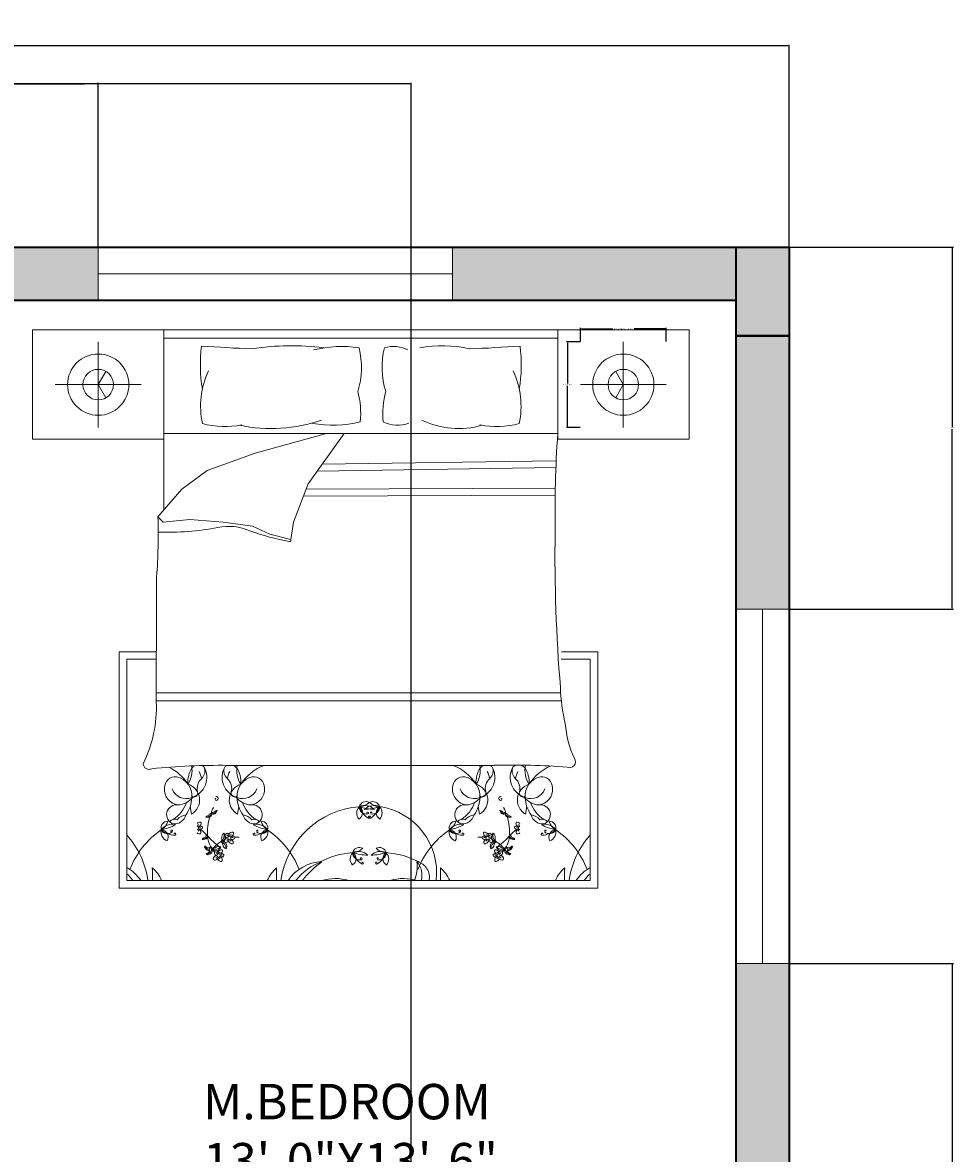
# Model space of a CAD drawing. Units: inches. Extents: x -10 to 455, y -513 to 57.
# Tile 4 of 4: x 297 to 455, y -134 to 57. Entities that reach past the tile are written whole.
import ezdxf

# ---------------------------------------------------------------- set-up
doc = ezdxf.new("R2010")
doc.units = ezdxf.units.IN
doc.header["$MEASUREMENT"] = 0
for name, color, linetype, lineweight in [('A-ANNO-DIMS', 2, 'Continuous', 18), ('A-AREA-IDEN', 7, 'Continuous', 18), ('A-COLS', 7, 'Continuous', 40), ('A-COLS-PATT', 1, 'Continuous', 13), ('A-FURN', 8, 'Continuous', 13), ('A-GLAZ', 222, 'Continuous', 18), ('A-WALL', 7, 'Continuous', 35), ('A-WALL-PATT', 152, 'Continuous', 13)]:
    doc.layers.add(name, color=color, linetype=linetype, lineweight=lineweight)
doc.styles.get("Standard").update_dxf_attribs({"font": 'arial.ttf'})
doc.dimstyles.get("Standard").update_dxf_attribs({"dimtxt": 0.18, "dimasz": 0.18, "dimexe": 0.18, "dimexo": 0.0625, "dimgap": 0.09, "dimtad": 0, "dimtih": 1, "dimtoh": 1, "dimdec": 0, "dimzin": 0, "dimdsep": 46, "dimlunit": 3, "dimtxsty": 'Standard', "dimcen": 0.09, "dimadec": 0, "dimazin": 0, "dimtfac": 1, "dimtdec": 0, "dimtofl": 0, "dimtmove": 0, "dimatfit": 3, "dimfxl": 1, "dimtolj": 1, "dimtzin": 0, "dimarcsym": 0})

# ---------------------------------------------------------------- blocks, each defined once
blk = doc.blocks.new('*D1')
at = {"layer": 'A-ANNO-DIMS', "color": 0, "lineweight": -2, "transparency": 16777216}
for p, q in [((40.25, 19.21), (40.25, 53.43)), ((40.43, 53.25), (223.35, 53.25)), ((427.07, 53.25), (244.14, 53.25)), ((427.25, 19.21), (427.25, 53.43))]:
    blk.add_line(p, q, dxfattribs=at)
at = {"layer": 'A-ANNO-DIMS', "color": 0, "transparency": 16777216}
for points in [[(40.43, 53.28), (40.43, 53.22), (40.25, 53.25)], [(427.07, 53.28), (427.07, 53.22), (427.25, 53.25)]]:
    blk.add_solid(points, dxfattribs=at)
at = {"layer": 'Defpoints', "color": 0, "transparency": 16777216}
for p in [(427.25, 53.25), (40.25, 19.15), (427.25, 19.15)]:
    blk.add_point(p, dxfattribs=at)
at = {"layer": 'A-ANNO-DIMS', "color": 0, "transparency": 16777216, "insert": (233.75, 53.25), "char_height": 6, "attachment_point": 5}
blk.add_mtext('\\A1;32\'-3"', dxfattribs=at)
blk = doc.blocks.new('WIN-60IN')
for p, q in [((0, 9), (60, 9)), ((0, 0), (0, 9)), ((60, 9), (60, 0)), ((0, 4.5), (60, 4.5)), ((60, 0), (0, 0))]:
    blk.add_line(p, q)
blk = doc.blocks.new('LAMP-BEDSIDE-LARGE')
for p, q in [((7.26, 0), (7.26, 14.53)), ((0, 7.26), (14.53, 7.26))]:
    blk.add_line(p, q)
for points in [[(7.26, 7.26), (5.97, 9.51)], [(7.26, 7.26), (5.97, 5.02)]]:
    blk.add_lwpolyline(points)
for radius in [5.19, 2.59]:
    blk.add_circle((7.26, 7.26), radius)
blk = doc.blocks.new('*D26')
at = {"layer": 'A-ANNO-DIMS', "color": 0, "lineweight": -2, "transparency": 16777216}
for p, q in [((391.92, 3.2), (391.92, 5.5)), ((392.1, 5.32), (397.38, 5.32)), ((406.27, 5.32), (401, 5.32)), ((406.45, 3.2), (406.45, 5.5))]:
    blk.add_line(p, q, dxfattribs=at)
at = {"layer": 'A-ANNO-DIMS', "color": 0, "transparency": 16777216}
for points in [[(392.1, 5.35), (392.1, 5.29), (391.92, 5.32)], [(406.27, 5.35), (406.27, 5.29), (406.45, 5.32)]]:
    blk.add_solid(points, dxfattribs=at)
at = {"layer": 'Defpoints', "color": 0, "transparency": 16777216}
for p in [(406.45, 5.32), (391.92, 3.14), (406.45, 3.14)]:
    blk.add_point(p, dxfattribs=at)
at = {"layer": 'A-ANNO-DIMS', "color": 0, "transparency": 16777216, "insert": (399.19, 5.32), "char_height": 0.18, "attachment_point": 5}
blk.add_mtext('\\A1;BEDSIDE LAMP 1\'-2 1/2" TYP.', dxfattribs=at)
blk = doc.blocks.new('*D27')
at = {"layer": 'A-ANNO-DIMS', "color": 0, "lineweight": -2, "transparency": 16777216}
for p, q in [((391.86, 3.14), (389.56, 3.14)), ((389.74, 2.96), (389.74, -3.94)), ((389.74, -11.21), (389.74, -4.31)), ((391.86, -11.39), (389.56, -11.39))]:
    blk.add_line(p, q, dxfattribs=at)
at = {"layer": 'A-ANNO-DIMS', "color": 0, "transparency": 16777216}
for points in [[(389.71, 2.96), (389.77, 2.96), (389.74, 3.14)], [(389.71, -11.21), (389.77, -11.21), (389.74, -11.39)]]:
    blk.add_solid(points, dxfattribs=at)
at = {"layer": 'Defpoints', "color": 0, "transparency": 16777216}
for p in [(389.74, 3.14), (391.92, 3.14), (391.92, -11.39)]:
    blk.add_point(p, dxfattribs=at)
at = {"layer": 'A-ANNO-DIMS', "color": 0, "transparency": 16777216, "insert": (389.74, -4.12), "char_height": 0.18, "attachment_point": 5}
blk.add_mtext('\\A1;1\'-2 1/2" TYP.', dxfattribs=at)
blk = doc.blocks.new('*D32')
at = {"layer": 'A-ANNO-DIMS', "color": 0, "lineweight": -2, "transparency": 16777216}
for p, q in [((237.5, 19.21), (237.5, 46.98)), ((237.68, 46.8), (273.54, 46.8)), ((310.07, 46.8), (274.2, 46.8)), ((310.25, 19.21), (310.25, 46.98))]:
    blk.add_line(p, q, dxfattribs=at)
at = {"layer": 'A-ANNO-DIMS', "color": 0, "transparency": 16777216}
for points in [[(237.68, 46.83), (237.68, 46.77), (237.5, 46.8)], [(310.07, 46.83), (310.07, 46.77), (310.25, 46.8)]]:
    blk.add_solid(points, dxfattribs=at)
at = {"layer": 'Defpoints', "color": 0, "transparency": 16777216}
for p in [(310.25, 46.8), (237.5, 19.15), (310.25, 19.15)]:
    blk.add_point(p, dxfattribs=at)
at = {"layer": 'A-ANNO-DIMS', "color": 0, "transparency": 16777216, "insert": (273.87, 46.8), "char_height": 0.18, "attachment_point": 5}
blk.add_mtext('\\A1;6\'-1"', dxfattribs=at)
blk = doc.blocks.new('*D37')
at = {"layer": 'A-ANNO-DIMS', "color": 0, "lineweight": -2, "transparency": 16777216}
for p, q in [((427.31, 19.15), (455.08, 19.15)), ((454.9, 18.97), (454.9, -11.33)), ((454.9, -41.99), (454.9, -11.69)), ((427.31, -42.17), (455.08, -42.17))]:
    blk.add_line(p, q, dxfattribs=at)
at = {"layer": 'A-ANNO-DIMS', "color": 0, "transparency": 16777216}
for points in [[(454.87, 18.97), (454.93, 18.97), (454.9, 19.15)], [(454.87, -41.99), (454.93, -41.99), (454.9, -42.17)]]:
    blk.add_solid(points, dxfattribs=at)
at = {"layer": 'Defpoints', "color": 0, "transparency": 16777216}
for p in [(427.25, 19.15), (427.25, -42.17), (454.9, -42.17)]:
    blk.add_point(p, dxfattribs=at)
at = {"layer": 'A-ANNO-DIMS', "color": 0, "transparency": 16777216, "insert": (454.9, -11.51), "char_height": 0.18, "attachment_point": 5}
blk.add_mtext('\\A1;5\'-1 1/2"', dxfattribs=at)
blk = doc.blocks.new('*D38')
at = {"layer": 'A-ANNO-DIMS', "color": 0, "lineweight": -2, "transparency": 16777216}
for p, q in [((427.31, -102.17), (455.08, -102.17)), ((454.9, -102.35), (454.9, -188.62)), ((454.9, -275.26), (454.9, -188.98)), ((427.31, -275.44), (455.08, -275.44))]:
    blk.add_line(p, q, dxfattribs=at)
at = {"layer": 'A-ANNO-DIMS', "color": 0, "transparency": 16777216}
for points in [[(454.87, -102.35), (454.93, -102.35), (454.9, -102.17)], [(454.87, -275.26), (454.93, -275.26), (454.9, -275.44)]]:
    blk.add_solid(points, dxfattribs=at)
at = {"layer": 'Defpoints', "color": 0, "transparency": 16777216}
for p in [(427.25, -102.17), (427.25, -275.44), (454.9, -275.44)]:
    blk.add_point(p, dxfattribs=at)
at = {"layer": 'A-ANNO-DIMS', "color": 0, "transparency": 16777216, "insert": (454.9, -188.8), "char_height": 0.18, "attachment_point": 5}
blk.add_mtext('\\A1;14\'-5 1/2"', dxfattribs=at)
blk = doc.blocks.new('*D41')
at = {"layer": 'A-ANNO-DIMS', "color": 0, "lineweight": -2, "transparency": 16777216}
for p, q in [((253.25, -160.79), (253.25, 46.98)), ((253.43, 46.8), (307.92, 46.8)), ((363.07, 46.8), (308.58, 46.8)), ((363.25, -160.79), (363.25, 46.98))]:
    blk.add_line(p, q, dxfattribs=at)
at = {"layer": 'A-ANNO-DIMS', "color": 0, "transparency": 16777216}
for points in [[(253.43, 46.83), (253.43, 46.77), (253.25, 46.8)], [(363.07, 46.83), (363.07, 46.77), (363.25, 46.8)]]:
    blk.add_solid(points, dxfattribs=at)
at = {"layer": 'Defpoints', "color": 0, "transparency": 16777216}
for p in [(363.25, 46.8), (253.25, -160.85), (363.25, -160.85)]:
    blk.add_point(p, dxfattribs=at)
at = {"layer": 'A-ANNO-DIMS', "color": 0, "transparency": 16777216, "insert": (308.25, 46.8), "char_height": 0.18, "attachment_point": 5}
blk.add_mtext('\\A1;9\'-2"', dxfattribs=at)
blk = doc.blocks.new('*D45')
at = {"layer": 'A-ANNO-DIMS', "color": 0, "lineweight": -2, "transparency": 16777216}
for p, q in [((257.66, -111.85), (257.84, -111.85)), ((257.75, -111.94), (257.75, -111.76)), ((300.74, -154.84), (284.74, -138.85)), ((300.92, -154.84), (300.74, -154.84))]:
    blk.add_line(p, q, dxfattribs=at)
at = {"layer": 'A-ANNO-DIMS', "color": 0, "transparency": 16777216}
blk.add_solid([(284.76, -138.83), (284.72, -138.87), (284.62, -138.72)], dxfattribs=at)
at = {"layer": 'Defpoints', "color": 0, "transparency": 16777216}
for p in [(257.75, -111.85), (284.62, -138.72)]:
    blk.add_point(p, dxfattribs=at)
at = {"layer": 'A-ANNO-DIMS', "color": 0, "transparency": 16777216, "insert": (301.33, -154.84), "char_height": 0.18, "attachment_point": 5}
blk.add_mtext('\\A1;R3\'-2"', dxfattribs=at)

msp = doc.modelspace()

# ---------------------------------------------------------------- hatches: boundary and pattern name
at = {"layer": 'A-COLS-PATT'}
h = msp.add_hatch(color=256, dxfattribs=at)
h.dxf.hatch_style = 1
h.paths.add_polyline_path([(55.25, 19.15), (40.25, 19.15), (40.25, 10.15), (55.25, 10.15)])
h.paths.add_polyline_path([(262.25, 19.15), (253.25, 19.15), (253.25, 4.15), (262.25, 4.15)])
h.paths.add_polyline_path([(427.25, 19.15), (418.25, 19.15), (418.25, 4.15), (427.25, 4.15)])
h.paths.add_polyline_path([(427.25, -247.85), (418.25, -247.85), (418.25, -262.85), (427.25, -262.85)])
h.paths.add_polyline_path([(268.25, -247.85), (253.25, -247.85), (253.25, -256.85), (268.25, -256.85)])
h.paths.add_polyline_path([(55.25, -247.85), (40.25, -247.85), (40.25, -256.85), (55.25, -256.85)])
h.paths.add_polyline_path([(55.25, -475.85), (49.25, -475.85), (40.25, -475.85), (40.25, -484.85), (55.25, -484.85)])
h.paths.add_polyline_path([(268.25, -475.85), (253.25, -475.85), (253.25, -484.85), (268.25, -484.85)])
h.paths.add_polyline_path([(427.25, -469.85), (418.25, -469.85), (418.25, -484.85), (427.25, -484.85)])
h.paths.add_polyline_path([(55.25, -100.85), (40.25, -100.85), (40.25, -109.85), (55.25, -109.85)])
at = {"layer": 'A-WALL-PATT'}
h = msp.add_hatch(color=256, dxfattribs=at)
h.dxf.hatch_style = 1
h.paths.add_polyline_path([(418.25, -151.85), (268.25, -151.85), (268.25, -160.85), (418.25, -160.85)])
h.paths.add_polyline_path([(165.25, -100.85), (55.25, -100.85), (55.25, -109.85), (165.25, -109.85), (165.25, -105.35)])
h.paths.add_polyline_path([(49.25, -75.35), (40.25, -75.35), (40.25, -100.85), (49.25, -100.85)])
h.paths.add_polyline_path([(49.25, 10.15), (40.25, 10.15), (40.25, -15.35), (49.25, -15.35)])
h.paths.add_polyline_path([(86.75, 19.15), (55.25, 19.15), (55.25, 10.15), (86.75, 10.15)])
h.paths.add_polyline_path([(213.5, 19.15), (146.75, 19.15), (146.75, 10.15), (193.25, 10.15), (193.25, -28.04), (197.75, -28.04), (197.75, 10.15), (213.5, 10.15)])
h.paths.add_polyline_path([(262.25, 4.15), (253.25, 4.15), (253.25, -69.35), (197.75, -69.35), (197.75, -60), (193.25, -60), (193.25, -109.85), (197.75, -109.85), (197.75, -73.85), (253.25, -73.85), (253.25, -109.85), (262.25, -109.85)])
h.paths.add_polyline_path([(310.25, 19.15), (262.25, 19.15), (262.25, 10.15), (310.25, 10.15)])
h.paths.add_polyline_path([(253.25, 19.15), (237.5, 19.15), (237.5, 10.15), (253.25, 10.15)])
h.paths.add_polyline_path([(418.25, 19.15), (370.25, 19.15), (370.25, 10.15), (418.25, 10.15)])
h.paths.add_polyline_path([(427.25, 4.15), (418.25, 4.15), (418.25, -42.17), (427.25, -42.17)])
h.paths.add_polyline_path([(427.25, -102.17), (418.25, -102.17), (418.25, -145.85), (427.25, -145.85)])
h.paths.add_polyline_path([(427.25, -160.85), (418.25, -160.85), (418.25, -247.85), (427.25, -247.85)])
h.paths.add_polyline_path([(418.25, -247.85), (365.75, -247.85), (365.75, -256.85), (418.25, -256.85)], flags=17)
h.paths.add_polyline_path([(297.25, -247.85), (268.25, -247.85), (268.25, -256.85), (297.25, -256.85), (297.25, -252.35)], flags=17)
h.paths.add_polyline_path([(427.25, -299.44), (418.25, -299.44), (418.25, -319.85), (370.25, -319.85), (370.25, -284.85), (368, -284.85), (365.75, -284.85), (365.75, -319.85), (329.75, -319.85), (329.75, -247.85), (325.25, -247.85), (325.25, -319.85), (257.75, -319.85), (257.75, -256.85), (253.25, -256.85), (253.25, -324.35), (262.25, -324.35), (418.25, -324.35), (418.25, -363.39), (427.25, -363.39)])
h.paths.add_polyline_path([(262.25, -352.35), (257.75, -352.35), (253.25, -352.35), (253.25, -447.85), (257.75, -447.85), (262.25, -447.85)])
h.paths.add_polyline_path([(305.75, -475.85), (268.25, -475.85), (268.25, -484.85), (305.75, -484.85)])
h.paths.add_polyline_path([(418.25, -475.85), (365.75, -475.85), (365.75, -484.85), (418.25, -484.85)])
h.paths.add_polyline_path([(427.25, -423.39), (418.25, -423.39), (418.25, -469.85), (427.25, -469.85)])
h.paths.add_polyline_path([(202.25, -247.85), (193.25, -247.85), (193.25, -403.85), (49.25, -403.85), (49.25, -360.35), (40.25, -360.35), (40.25, -412.85), (202.25, -412.85)])
h.paths.add_polyline_path([(165.25, -247.85), (55.25, -247.85), (55.25, -256.85), (165.25, -256.85), (165.25, -252.35)], flags=17)
h.paths.add_polyline_path([(49.25, -225.11), (40.25, -225.11), (40.25, -247.85), (49.25, -247.85)])
h.paths.add_polyline_path([(49.25, -256.85), (40.25, -256.85), (40.25, -300.35), (49.25, -300.35)], flags=17)
h.paths.add_polyline_path([(49.25, -137.85), (44.75, -137.85), (40.25, -137.85), (40.25, -165.11), (49.25, -165.11)])

# ---------------------------------------------------------------- linework, layer by layer
at = {"layer": 'A-COLS'}
msp.add_line((418.25, 4.15), (427.25, 4.15), dxfattribs=at)
at = {"layer": 'A-FURN'}
for p, q in [((299.12, 5.14), (410.31, 5.14)), ((321.35, 5.14), (321.35, -25.38)), ((388.07, 3.72), (321.35, 3.72)), ((321.35, -12.43), (388.07, -12.43)), ((336.8, -15.73), (348.92, -12.43)), ((351.9, -12.43), (345.81, -20.91)), ((328.69, -18.66), (336.8, -15.73)), ((387.77, -17.05), (348.18, -17.6)), ((324.41, -21.81), (328.69, -18.66)), ((387.73, -18.19), (347.35, -18.76)), ((345.81, -20.91), (343.33, -27.44)), ((320.36, -26.54), (324.41, -21.81)), ((387.68, -22.83), (345.01, -23.01)), ((387.67, -21.69), (345.45, -21.86)), ((321.26, -27.44), (320.36, -26.54)), ((325.76, -26.99), (321.26, -27.44)), ((331.39, -27.44), (325.76, -26.99)), ((336.35, -28.11), (331.39, -27.44)), ((339.28, -29.46), (336.35, -28.11)), ((343.33, -27.44), (342.88, -30.36)), ((342.88, -30.36), (339.28, -29.46)), ((313.79, -49.36), (320.08, -49.36)), ((313.79, -89.42), (313.79, -49.36)), ((388.69, -49.36), (394.86, -49.36)), ((394.86, -49.36), (394.86, -89.42)), ((320.08, -50.65), (315.08, -50.65)), ((315.08, -50.65), (315.08, -88.13)), ((393.57, -50.65), (388.67, -50.65)), ((393.57, -88.13), (393.57, -50.65)), ((388.57, -56.3), (320.07, -56.3)), ((388.68, -57.69), (320.07, -57.69)), ((377.28, -68.61), (332.14, -68.61)), ((326.04, -76.86), (325.79, -75.6)), ((333.81, -76.86), (334.05, -75.6)), ((374.84, -76.86), (374.59, -75.6)), ((382.61, -76.86), (382.86, -75.6)), ((394.86, -89.42), (313.79, -89.42)), ((315.08, -88.13), (393.57, -88.13))]:
    msp.add_line(p, q, dxfattribs=at)
for points in [[(321.35, -13.39), (299.12, -13.39), (299.12, 5.14)], [(388.07, 5.14), (388.07, -13.39), (410.31, -13.39), (410.31, 5.14)]]:
    msp.add_lwpolyline(points, dxfattribs=at)
for points in [[(327.74, 2.37, 0.074897), (327.88, -4.89, -0.472817)], [(354.19, -5.3, 0.14099), (354.41, 2.11, 0.235245)], [(358.94, -5.3, -0.14099), (358.72, 2.11, -0.235245)], [(381.68, 2.37, -0.074897), (381.55, -4.89, 0.472817)], [(320.13, -36.72, 0.001242), (320.07, -57.82, -0.127202), (317.84, -68.33)], [(388.54, -55.42, 0.056112), (389.35, -61.54, 0.095341), (390.91, -67.43)]]:
    msp.add_lwpolyline(points, format="xyb", dxfattribs=at)
for centre in [(332.46, -80.89), (376.19, -80.89), (330.61, -83.87), (378.04, -83.87)]:
    msp.add_circle(centre, 0.283, dxfattribs=at)
for centre, radius, start, end in [((389.03, 1060.56), 1059.96, 266.68521, 267.14978), ((342.98, -37.86), 40.33, 82.2196, 99.497), ((351.49, -17.48), 19.81, 81.5249, 103.96), ((360.24, -3.17), 5.5, 63.3437, 106.1026), ((368.49, -17.08), 19.55, 76.3427, 101.1841), ((320.39, 1060.56), 1059.96, 272.85022, 273.31479), ((341.91, -7.81), 14.33, 155.1316, 191.7583), ((367.52, -7.81), 14.33, 348.2417, 24.8684), ((341.08, -9.01), 13.62, 354.0129, 15.8293), ((372.05, -9.01), 13.62, 164.1707, 185.9871), ((331.71, 3.67), 14.9, 255.1039, 281.0369), ((339.55, 14.27), 25.84, 258.0397, 289.2615), ((350.01, 8.62), 19.61, 259.8617, 283.6238), ((360.99, -5.09), 5.89, 245.0183, 288.5407), ((371.29, 2.58), 14.15, 243.8761, 286.1746), ((377.72, 3.67), 14.9, 258.9631, 284.8961), ((587.4, -26.02), 199.79, 176.1, 180.9282), ((218.41, -29.3), 101.99, 355.8294, 1.553), ((322.26, 12.84), 41.97, 267.4519, 281.3392), ((332.29, -37.18), 9.05, 66.2616, 101.3392), ((350.6, 11.66), 43.12, 250.1194, 259.3383), ((342.63, -30.45), 0.268, 268.8623, 19.7536), ((648.22, -33.28), 260.62, 179.1145, 184.8735), ((318.87, -68.26), 1.03, 183.98, 297.3412), ((330.81, -184.35), 115.75, 89.3433, 95.6887), ((318.43, -76.44), 8.42, 33.6671, 63.2997), ((321.52, -69.43), 4.61, 328.8218, 9.1554), ((327.23, -69.84), 1.34, 120.0293, 142.325), ((325.09, -70.63), 3.54, 289.2822, 29.1751), ((326.66, -69.57), 1.66, 311.5653, 23.8354), ((327.23, -69.84), 1.34, 44.4517, 63.558), ((334.76, -70.63), 3.54, 150.8249, 250.7178), ((333.19, -69.57), 1.66, 156.1646, 228.4347), ((332.62, -69.84), 1.34, 113.229, 135.5483), ((332.62, -69.84), 1.34, 37.675, 66.7144), ((338.33, -69.43), 4.61, 169.7133, 211.1782), ((341.41, -76.44), 8.42, 111.4941, 146.3329), ((367.23, -76.44), 8.42, 33.6671, 68.5059), ((370.32, -69.43), 4.61, 328.8218, 10.2867), ((376.03, -69.84), 1.34, 113.2856, 142.325), ((373.89, -70.63), 3.54, 289.2822, 29.1751), ((376.03, -69.84), 1.34, 44.4517, 66.7144), ((375.46, -69.57), 1.66, 311.5653, 23.8354), ((380.69, -176.75), 108.2, 85.2402, 91.8035), ((383.56, -70.63), 3.54, 150.8249, 250.7178), ((381.99, -69.57), 1.66, 156.1646, 228.4347), ((381.42, -69.84), 1.34, 106.6343, 135.5483), ((381.42, -69.84), 1.34, 37.675, 72.5814), ((387.13, -69.43), 4.61, 169.249, 211.1782), ((390.21, -76.44), 8.42, 113.6453, 146.3329), ((390.07, -68), 1.01, 246.5219, 33.8264), ((323.34, -72.4), 1.88, 84.4856, 181.0538), ((322.76, -73.79), 3.34, 355.2933, 76.921), ((329.71, -71.43), 4.29, 145.785, 184.7304), ((329.28, -72.52), 2.28, 131.5653, 195.1471), ((324.55, -71.27), 3.2, 7.436, 29.9149), ((330.57, -72.52), 2.28, 344.8529, 48.4347), ((335.29, -71.27), 3.2, 150.0851, 172.564), ((330.13, -71.43), 4.29, 355.2696, 34.215), ((337.09, -73.79), 3.34, 103.079, 184.7067), ((336.51, -72.4), 1.88, 358.9462, 95.5144), ((372.14, -72.4), 1.88, 84.4856, 181.0538), ((371.56, -73.79), 3.34, 355.2933, 76.921), ((378.51, -71.43), 4.29, 145.785, 184.7304), ((378.08, -72.52), 2.28, 131.5653, 195.1471), ((373.35, -71.27), 3.2, 7.436, 29.9149), ((379.37, -72.52), 2.28, 344.8529, 48.4347), ((384.09, -71.27), 3.2, 150.0851, 172.564), ((378.94, -71.43), 4.29, 355.2696, 34.215), ((385.89, -73.79), 3.34, 103.079, 184.7067), ((385.31, -72.4), 1.88, 358.9462, 95.5144), ((324.11, -72.67), 2.66, 174.9449, 262.8857), ((325.15, -71.66), 2.58, 201.5819, 291.4221), ((324.66, -74.46), 2.76, 299.9085, 73.1337), ((335.19, -74.46), 2.76, 106.8663, 240.0915), ((334.7, -71.66), 2.58, 248.5779, 338.4181), ((335.74, -72.67), 2.66, 277.1143, 5.0551), ((372.91, -72.67), 2.66, 174.9449, 262.8857), ((373.95, -71.66), 2.58, 201.5819, 291.4221), ((373.46, -74.46), 2.76, 299.9085, 73.1337), ((383.99, -74.46), 2.76, 106.8663, 240.0915), ((383.5, -71.66), 2.58, 248.5779, 338.4181), ((384.54, -72.67), 2.66, 277.1143, 5.0551), ((323.64, -72.08), 3.23, 272.3591, 324.0401), ((320.14, -73.7), 5.97, 326.2883, 356.5076), ((329.71, -71.43), 4.29, 212.7011, 216.3445), ((326.41, -73.3), 0.69, 257.3041, 15.1471), ((330.24, -74.35), 0.214, 102.7051, 280.4384), ((330.22, -74.21), 0.348, 280.4384, 100.4136), ((333.44, -73.3), 0.69, 164.8529, 282.6959), ((330.13, -71.43), 4.29, 323.6555, 327.2989), ((336.2, -72.08), 3.23, 215.9599, 267.6409), ((339.71, -73.7), 5.97, 183.4924, 213.7117), ((372.44, -72.08), 3.23, 272.3591, 324.0401), ((368.94, -73.7), 5.97, 326.2883, 356.5076), ((378.51, -71.43), 4.29, 212.7011, 216.3445), ((375.21, -73.3), 0.69, 257.3041, 15.1471), ((378.43, -74.21), 0.348, 79.5864, 259.5616), ((378.41, -74.35), 0.214, 259.5616, 77.2949), ((382.24, -73.3), 0.69, 164.8529, 282.6959), ((378.94, -71.43), 4.29, 323.6555, 327.2989), ((385, -72.08), 3.23, 215.9599, 267.6409), ((388.51, -73.7), 5.97, 183.4924, 213.7117), ((323.49, -76.95), 1.67, 80.264, 250.8688), ((320.19, -73.27), 5.25, 301.2614, 341.7045), ((337.95, -79.94), 9.21, 153.0032, 159.8941), ((329.65, -76.79), 0.227, 84.3784, 186.0543), ((329.19, -74.84), 1.79, 285.5129, 293.6099), ((330.36, -76.85), 0.584, 87.3579, 140.4944), ((329.01, -75.18), 1.76, 301.164, 321.5612), ((327.58, -74.87), 3.14, 324.6898, 333.4936), ((339.66, -73.27), 5.25, 198.2955, 238.7386), ((336.35, -76.95), 1.67, 289.1312, 99.736), ((355.58, -90.09), 14.52, 94.4623, 172.255), ((355.64, -76.69), 1.61, 137.7873, 219.1145), ((353.81, -76.64), 1.21, 298.5391, 58.3627), ((355.6, -75.95), 1.2, 63.0274, 163.8037), ((354.38, -73.13), 2.48, 271.4585, 315.3727), ((355.39, -77.7), 2.3, 45.5411, 114.3101), ((357.49, -65.92), 10.16, 252.593, 267.2582), ((355.63, -75.66), 1.19, 177.7585, 283.852), ((357.92, -74.42), 3.67, 198.9159, 238.011), ((356.96, -77.7), 2.3, 65.6899, 134.4589), ((354.87, -65.92), 10.16, 272.7418, 287.407), ((355.88, -76.66), 0.157, 283.852, 219.9245), ((356.75, -75.95), 1.2, 16.1963, 116.9726), ((357.97, -73.13), 2.48, 224.6273, 268.5415), ((356.46, -76.6), 0.0947, 320.1909, 256.0209), ((354.43, -74.42), 3.67, 301.989, 341.0841), ((356.72, -75.66), 1.19, 256.148, 2.2415), ((358.54, -76.64), 1.21, 121.6373, 241.4609), ((356.71, -76.69), 1.61, 320.8855, 42.2127), ((356.31, -86.73), 11.24, 352.8636, 81.8197), ((372.3, -76.95), 1.67, 80.264, 250.8688), ((368.99, -73.27), 5.25, 301.2614, 341.7045), ((379.64, -75.18), 1.76, 218.4388, 238.836), ((378.29, -76.85), 0.584, 39.5056, 92.6421), ((381.07, -74.87), 3.14, 206.5064, 215.3102), ((379.45, -74.84), 1.79, 246.3901, 254.4871), ((370.7, -79.94), 9.21, 20.1059, 26.9968), ((379, -76.79), 0.227, 353.9457, 95.6216), ((388.46, -73.27), 5.25, 198.2955, 238.7386), ((385.15, -76.95), 1.67, 289.1312, 99.736), ((322.08, -79.25), 1.2, 92.9516, 193.728), ((319.62, -77.42), 2.48, 301.3827, 345.2969), ((323.15, -78.76), 1.02, 63.9755, 143.2681), ((323.09, -76.44), 2.08, 265.969, 344.3045), ((325.34, -79.22), 2.22, 96.1662, 141.5825), ((327.36, -78.76), 0.472, 101.5637, 142.6358), ((326.98, -78.39), 0.681, 288.7263, 352.5032), ((327.45, -78.43), 0.219, 345.2356, 144.9248), ((329.01, -77.66), 0.584, 101.3256, 154.4621), ((328.17, -75.68), 1.76, 280.2588, 300.656), ((328.58, -74.27), 3.14, 268.3264, 277.1302), ((337.95, -79.94), 9.21, 163.5842, 183.8277), ((327.79, -75.68), 1.79, 308.2101, 316.3071), ((328.89, -76.86), 0.534, 278.3432, 4.2869), ((328.6, -76.39), 0.932, 300.656, 332.6341), ((329.3, -77), 0.227, 55.7657, 157.4417), ((329.44, -75.88), 0.932, 269.1859, 301.164), ((329.71, -76.37), 0.534, 237.5332, 323.4768), ((334.51, -79.22), 2.22, 38.4175, 83.8338), ((336.75, -76.44), 2.08, 195.6955, 274.031), ((336.7, -78.76), 1.02, 36.7319, 116.0245), ((337.77, -79.25), 1.2, 346.272, 87.0484), ((340.23, -77.42), 2.48, 194.7031, 238.6173), ((356.07, -77.38), 0.18, 238.011, 71.5592), ((356.1, -77.29), 0.0876, 71.5592, 188.0167), ((356.28, -77.38), 0.18, 108.4408, 301.989), ((356.25, -77.29), 0.0876, 351.9833, 108.4408), ((370.88, -79.25), 1.2, 92.9516, 193.728), ((368.42, -77.42), 2.48, 301.3827, 345.2969), ((371.95, -78.76), 1.02, 63.9755, 143.2681), ((371.9, -76.44), 2.08, 265.969, 344.3045), ((374.14, -79.22), 2.22, 96.1662, 141.5825), ((378.94, -76.37), 0.534, 216.5232, 302.4668), ((379.21, -75.88), 0.932, 238.836, 270.8141), ((379.35, -77), 0.227, 22.5583, 124.2343), ((379.76, -76.86), 0.534, 175.7131, 261.6568), ((380.05, -76.39), 0.932, 207.3659, 239.344), ((370.7, -79.94), 9.21, 356.1723, 16.4158), ((380.85, -75.68), 1.79, 223.6929, 231.7899), ((380.47, -75.68), 1.76, 239.344, 259.7412), ((380.07, -74.27), 3.14, 262.8698, 271.6736), ((379.63, -77.66), 0.584, 25.5379, 78.6744), ((381.2, -78.43), 0.219, 35.0752, 194.7644), ((381.66, -78.39), 0.681, 187.4968, 251.2737), ((381.28, -78.76), 0.472, 37.3642, 78.4363), ((385.55, -76.44), 2.08, 195.6955, 274.031), ((383.31, -79.22), 2.22, 38.4175, 83.8338), ((385.5, -78.76), 1.02, 36.7319, 116.0245), ((389.03, -77.42), 2.48, 194.7031, 238.6173), ((386.57, -79.25), 1.2, 346.272, 87.0484), ((304.27, -90.09), 14.52, 7.745, 41.8856), ((329.11, -91.52), 14.52, 124.3865, 158.5908), ((322.48, -79.88), 1.61, 167.7115, 249.0387), ((322.77, -80.88), 2.3, 75.4653, 144.2343), ((318.71, -69.62), 10.16, 282.5173, 297.1824), ((320.88, -80.75), 1.21, 328.4633, 88.2869), ((323.33, -76.77), 3.67, 228.8402, 267.9352), ((321.96, -78.99), 1.19, 207.6827, 313.7762), ((322.68, -79.73), 0.157, 313.7762, 249.7183), ((323.18, -80.17), 0.0876, 101.4834, 217.9409), ((323.2, -80.26), 0.18, 267.9352, 101.4834), ((326.97, -79.2), 0.283, 273.2768, 86.7232), ((327.36, -79.73), 0.468, 217.7621, 259.0403), ((327.3, -78.93), 0.27, 91.1081, 181.8675), ((327.86, -79.1), 0.86, 203.4276, 227.6104), ((327.59, -79.48), 0.585, 80.3487, 133.6538), ((327.48, -78.99), 0.463, 229.7889, 317.6792), ((326.96, -79.98), 0.658, 355.053, 68.3618), ((327.48, -80.09), 0.927, 83.0852, 105.7171), ((327.4, -80.01), 0.217, 232.4737, 355.053), ((321.06, -87.78), 10.56, 43.1541, 52.0459), ((327.65, -79.14), 0.244, 317.6792, 80.3487), ((330.29, -80.46), 1.29, 304.5369, 16.3699), ((332.09, -80.83), 0.913, 127.3105, 187.9252), ((330.83, -80.72), 0.938, 355.0106, 41.658), ((332.15, -80.49), 0.386, 126.1046, 271.4281), ((332.11, -80.39), 0.277, 353.7526, 131.7054), ((331.85, -80.72), 0.39, 0.0645, 61.1507), ((331.94, -80.38), 0.445, 311.8413, 355.7877), ((332.85, -80.45), 0.472, 101.5637, 176.365), ((332.79, -80.62), 0.27, 91.1081, 181.8675), ((332.47, -80.08), 0.681, 288.7263, 352.5032), ((332.94, -80.11), 0.219, 345.2356, 144.9248), ((336.64, -80.26), 0.18, 78.5166, 272.0648), ((337.07, -80.88), 2.3, 35.7657, 104.5347), ((341.14, -69.62), 10.16, 242.8176, 257.4827), ((336.52, -76.77), 3.67, 272.0648, 311.1598), ((336.66, -80.17), 0.0876, 322.0591, 78.5166), ((337.88, -78.99), 1.19, 226.2238, 332.3173), ((337.19, -79.67), 0.0947, 290.2667, 226.2271), ((338.97, -80.75), 1.21, 91.7131, 211.5367), ((337.36, -79.88), 1.61, 290.9613, 12.2885), ((330.73, -91.52), 14.52, 21.4092, 55.6135), ((377.91, -91.52), 14.52, 124.3865, 158.5908), ((371.29, -79.88), 1.61, 167.7115, 249.0387), ((371.58, -80.88), 2.3, 75.4653, 144.2343), ((367.51, -69.62), 10.16, 282.5173, 297.1824), ((370.76, -78.99), 1.19, 207.6827, 313.7762), ((372.13, -76.77), 3.67, 228.8402, 267.9352), ((369.68, -80.75), 1.21, 328.4633, 88.2869), ((371.48, -79.73), 0.157, 313.7762, 249.7183), ((371.99, -80.17), 0.0876, 101.4834, 217.9409), ((372, -80.26), 0.18, 267.9352, 101.4834), ((375.71, -80.11), 0.219, 35.0752, 194.7644), ((376.17, -80.08), 0.681, 187.4968, 251.2737), ((375.86, -80.62), 0.27, 358.1325, 88.8919), ((375.79, -80.45), 0.472, 3.635, 78.4363), ((376.54, -80.39), 0.277, 48.2946, 186.2474), ((376.71, -80.38), 0.445, 184.2123, 228.1587), ((376.8, -80.72), 0.39, 118.8493, 179.9355), ((376.5, -80.49), 0.386, 268.5719, 53.8954), ((377.82, -80.72), 0.938, 138.342, 184.9894), ((378.35, -80.46), 1.29, 163.6301, 235.4631), ((376.56, -80.83), 0.913, 352.0748, 52.6895), ((387.59, -87.78), 10.56, 127.9541, 136.8459), ((381, -79.14), 0.244, 99.6513, 222.3208), ((381.16, -78.99), 0.463, 222.3208, 310.2111), ((381.06, -79.48), 0.585, 46.3462, 99.6513), ((381.69, -79.98), 0.658, 111.6382, 184.947), ((381.25, -80.01), 0.217, 184.947, 307.5263), ((381.17, -80.09), 0.927, 74.2829, 96.9148), ((381.35, -78.93), 0.27, 358.1325, 88.8919), ((380.78, -79.1), 0.86, 312.3896, 336.5724), ((381.29, -79.73), 0.468, 280.9597, 322.2379), ((381.68, -79.2), 0.283, 93.2768, 266.7232), ((385.44, -80.26), 0.18, 78.5166, 272.0648), ((385.87, -80.88), 2.3, 35.7657, 104.5347), ((389.94, -69.62), 10.16, 242.8176, 257.4827), ((385.32, -76.77), 3.67, 272.0648, 311.1598), ((385.46, -80.17), 0.0876, 322.0591, 78.5166), ((386.68, -78.99), 1.19, 226.2238, 332.3173), ((385.99, -79.67), 0.0947, 290.2667, 226.2271), ((387.77, -80.75), 1.21, 91.7131, 211.5367), ((386.16, -79.88), 1.61, 290.9613, 12.2885), ((379.54, -91.52), 14.52, 21.4092, 55.6135), ((404.38, -90.09), 14.52, 138.1144, 172.255), ((328.35, -81.4), 0.584, 101.3256, 154.4621), ((327.51, -79.42), 1.76, 280.2588, 300.656), ((327.92, -78.01), 3.14, 268.3264, 277.1302), ((328.55, -82.42), 0.316, 146.8636, 236.9021), ((327.13, -79.42), 1.79, 308.2101, 316.3071), ((333.01, -75.46), 8.27, 235.1882, 238.8844), ((329.09, -81.97), 0.856, 199.4799, 267.6828), ((328.23, -80.6), 0.534, 278.3432, 4.2869), ((327.93, -80.13), 0.932, 300.656, 332.6341), ((328.63, -80.74), 0.227, 55.7657, 157.4417), ((333.36, -80.17), 4.62, 184.756, 209.2041), ((340.01, -70.34), 15.19, 222.2412, 232.1744), ((333.84, -86.31), 5.54, 120.544, 139.818), ((330.68, -83.26), 0.913, 70.0041, 130.6188), ((330.98, -80.75), 0.785, 272.8499, 356.1226), ((330.43, -81.06), 0.76, 321.7607, 7.9252), ((330.59, -82.15), 0.76, 8.7227, 54.8872), ((330.63, -82.76), 1.29, 0.278, 72.111), ((331.21, -82.28), 0.785, 20.5253, 88.5375), ((332.24, -81.9), 0.913, 188.7227, 249.3375), ((331.87, -81.42), 0.281, 148.0499, 225.6268), ((333.84, -86.31), 5.54, 113.0501, 113.8477), ((332.39, -81.74), 0.893, 104.7558, 148.0499), ((331.89, -81.1), 0.559, 247.4086, 351.4386), ((331.07, -82.35), 0.938, 334.9899, 21.6373), ((332.04, -81.12), 0.188, 262.906, 7.132), ((332.85, -81.41), 0.468, 151.2196, 259.0403), ((333.35, -80.79), 0.86, 203.4276, 227.6104), ((333.08, -81.16), 0.585, 80.3487, 133.6538), ((332.97, -80.68), 0.463, 229.7889, 317.6792), ((332.45, -81.66), 0.658, 355.053, 68.3618), ((332.97, -81.77), 0.927, 83.0852, 105.7171), ((332.89, -81.7), 0.217, 232.4737, 355.053), ((333.14, -80.83), 0.244, 317.6792, 80.3487), ((333.84, -86.31), 5.54, 87.1071, 94.7585), ((374.81, -86.31), 5.54, 85.2415, 92.8929), ((375.51, -80.83), 0.244, 99.6513, 222.3208), ((375.67, -80.68), 0.463, 222.3208, 310.2111), ((375.57, -81.16), 0.585, 46.3462, 99.6513), ((376.2, -81.66), 0.658, 111.6382, 184.947), ((375.76, -81.7), 0.217, 184.947, 307.5263), ((375.68, -81.77), 0.927, 74.2829, 96.9148), ((375.3, -80.79), 0.86, 312.3896, 336.5724), ((375.8, -81.41), 0.468, 280.9597, 28.7804), ((376.76, -81.1), 0.559, 188.5614, 292.5914), ((376.61, -81.12), 0.188, 172.868, 277.094), ((376.26, -81.74), 0.893, 31.9501, 75.2442), ((377.58, -82.35), 0.938, 158.3627, 205.0101), ((377.44, -82.28), 0.785, 91.4625, 159.4747), ((378.02, -82.76), 1.29, 107.889, 179.722), ((376.41, -81.9), 0.913, 290.6625, 351.2773), ((377.66, -80.75), 0.785, 183.8774, 267.1501), ((374.81, -86.31), 5.54, 66.1523, 66.9499), ((376.78, -81.42), 0.281, 314.3732, 31.9501), ((378.06, -82.15), 0.76, 125.1128, 171.2773), ((378.22, -81.06), 0.76, 172.0748, 218.2393), ((374.81, -86.31), 5.54, 40.182, 59.456), ((377.97, -83.26), 0.913, 49.3812, 109.9959), ((368.64, -70.34), 15.19, 307.8256, 317.7588), ((375.29, -80.17), 4.62, 330.7959, 355.244), ((379.56, -81.97), 0.856, 272.3172, 340.5201), ((380.01, -80.74), 0.227, 22.5583, 124.2343), ((380.42, -80.6), 0.534, 175.7131, 261.6568), ((380.71, -80.13), 0.932, 207.3659, 239.344), ((375.64, -75.46), 8.27, 301.1156, 304.8118), ((381.52, -79.42), 1.79, 223.6929, 231.7899), ((381.14, -79.42), 1.76, 239.344, 259.7412), ((380.1, -82.42), 0.316, 303.0979, 33.1364), ((380.73, -78.01), 3.14, 262.8698, 271.6736), ((380.3, -81.4), 0.584, 25.5379, 78.6744), ((329, -82.29), 0.737, 212.8155, 277.3992), ((328.57, -82.78), 0.856, 266.9701, 338.2913), ((324.06, -76.67), 8.27, 302.6784, 306.3746), ((328.78, -83.46), 0.316, 214.3538, 304.3923), ((328.9, -82.26), 0.327, 238.8844, 314.2646), ((328.83, -82.99), 0.737, 280.3057, 17.1958), ((328.77, -83.07), 0.327, 306.3746, 21.7548), ((329.3, -82.86), 0.247, 19.3605, 201.7548), ((329.3, -82.67), 0.247, 311.8703, 134.2646), ((333.94, -84.92), 4.93, 153.7819, 158.2913), ((330.02, -81.55), 1.29, 247.2305, 319.0635), ((329.59, -81.99), 0.76, 264.4544, 310.6188), ((333.36, -80.17), 4.62, 214.0033, 222.4917), ((330.15, -82.29), 0.785, 218.3208, 298.8162), ((330.01, -84.4), 0.281, 148.0499, 225.6268), ((330.53, -84.73), 0.893, 104.7558, 148.0499), ((330.03, -84.09), 0.559, 247.4086, 351.4386), ((330.3, -83.48), 0.386, 126.1046, 271.4281), ((330.25, -83.37), 0.277, 353.7526, 131.7054), ((330.19, -84.11), 0.188, 262.906, 7.132), ((329.99, -83.7), 0.39, 0.0645, 61.1507), ((330.09, -83.37), 0.445, 311.8413, 355.7877), ((330.09, -82.15), 0.938, 297.7043, 344.3516), ((331, -83.43), 0.472, 101.5637, 176.365), ((331, -84.39), 0.468, 151.2196, 259.0403), ((330.94, -83.6), 0.27, 91.1081, 181.8675), ((331.5, -83.77), 0.86, 203.4276, 227.6104), ((331.23, -84.15), 0.585, 80.3487, 133.6538), ((331.12, -83.66), 0.463, 229.7889, 317.6792), ((330.62, -83.06), 0.681, 288.7263, 352.5032), ((330.6, -84.64), 0.658, 355.053, 68.3618), ((331.12, -84.76), 0.927, 83.0852, 105.7171), ((331.09, -83.1), 0.219, 345.2356, 144.9248), ((331.28, -83.81), 0.244, 317.6792, 80.3487), ((354.46, -97.86), 14.52, 94.4623, 117.4146), ((354.53, -84.47), 1.61, 137.7873, 219.1145), ((352.7, -84.42), 1.21, 298.5391, 58.3627), ((354.49, -83.72), 1.2, 63.0274, 163.8037), ((353.27, -80.91), 2.48, 271.4585, 315.3727), ((354.28, -85.48), 2.3, 45.5411, 114.3101), ((356.81, -82.2), 3.67, 198.9159, 238.011), ((356.37, -73.69), 10.16, 252.593, 267.2582), ((354.52, -83.43), 1.19, 177.7585, 283.852), ((358.07, -85.48), 2.3, 65.6899, 134.4589), ((355.98, -73.69), 10.16, 272.7418, 287.407), ((357.86, -83.72), 1.2, 16.1963, 116.9726), ((359.08, -80.91), 2.48, 224.6273, 268.5415), ((355.55, -82.2), 3.67, 301.989, 341.0841), ((357.83, -83.43), 1.19, 256.148, 2.2415), ((359.66, -84.42), 1.21, 121.6373, 241.4609), ((357.83, -84.47), 1.61, 320.8855, 42.2127), ((357.89, -97.86), 14.52, 62.5854, 85.5377), ((377.36, -83.81), 0.244, 99.6513, 222.3208), ((377.53, -83.66), 0.463, 222.3208, 310.2111), ((377.42, -84.15), 0.585, 46.3462, 99.6513), ((377.56, -83.1), 0.219, 35.0752, 194.7644), ((378.03, -83.06), 0.681, 187.4968, 251.2737), ((378.05, -84.64), 0.658, 111.6382, 184.947), ((377.53, -84.76), 0.927, 74.2829, 96.9148), ((378.63, -81.55), 1.29, 220.9365, 292.7695), ((378.56, -82.15), 0.938, 195.6484, 242.2957), ((377.71, -83.6), 0.27, 358.1325, 88.8919), ((377.15, -83.77), 0.86, 312.3896, 336.5724), ((377.65, -83.43), 0.472, 3.635, 78.4363), ((377.65, -84.39), 0.468, 280.9597, 28.7804), ((378.61, -84.09), 0.559, 188.5614, 292.5914), ((378.5, -82.29), 0.785, 241.1838, 321.6792), ((378.39, -83.37), 0.277, 48.2946, 186.2474), ((378.56, -83.37), 0.445, 184.2123, 228.1587), ((378.65, -83.7), 0.39, 118.8493, 179.9355), ((378.46, -84.11), 0.188, 172.868, 277.094), ((378.35, -83.48), 0.386, 268.5719, 53.8954), ((378.11, -84.73), 0.893, 31.9501, 75.2442), ((379.05, -81.99), 0.76, 229.3812, 275.5456), ((375.29, -80.17), 4.62, 317.5083, 325.9967), ((378.63, -84.4), 0.281, 314.3732, 31.9501), ((379.82, -82.99), 0.737, 162.8042, 259.6943), ((379.35, -82.67), 0.247, 45.7354, 228.1297), ((379.35, -82.86), 0.247, 338.2452, 160.6395), ((374.7, -84.92), 4.93, 21.7087, 26.2181), ((380.08, -82.78), 0.856, 201.7087, 273.0299), ((379.75, -82.26), 0.327, 225.7354, 301.1156), ((379.88, -83.07), 0.327, 158.2452, 233.6254), ((379.65, -82.29), 0.737, 262.6008, 327.1845), ((384.59, -76.67), 8.27, 233.6254, 237.3216), ((379.86, -83.46), 0.316, 235.6077, 325.6462), ((311.55, -92.03), 7.08, 33.4617, 60.1116), ((315.52, -90.39), 5.9, 22.5547, 48.9546), ((299.35, -87.22), 20.09, 357.4081, 3.6519), ((331.04, -84.68), 0.217, 232.4737, 355.053), ((344.33, -90.39), 5.9, 131.0454, 157.4453), ((360.5, -87.22), 20.09, 176.3481, 182.5919), ((348.29, -92.03), 7.08, 91.272, 146.5383), ((350.84, -93.35), 8.82, 107.8504, 143.6964), ((355.47, -95.83), 13.12, 124.0123, 144.053), ((354.77, -84.43), 0.157, 283.852, 219.9245), ((354.96, -85.16), 0.18, 238.011, 71.5592), ((354.99, -85.07), 0.0876, 71.5592, 188.0167), ((357.4, -85.16), 0.18, 108.4408, 301.989), ((357.37, -85.07), 0.0876, 351.9833, 108.4408), ((357.57, -84.37), 0.0947, 320.1909, 256.0209), ((357.76, -85.71), 6.5, 338.117, 6.6195), ((363.73, -87.52), 2.61, 346.3898, 79.0739), ((361.77, -87.16), 3.3, 342.8609, 41.9049), ((348.15, -87.22), 20.09, 357.4081, 3.6519), ((364.32, -90.39), 5.9, 22.5547, 48.9546), ((377.61, -84.68), 0.217, 184.947, 307.5263), ((393.13, -90.39), 5.9, 131.0454, 157.4453), ((409.3, -87.22), 20.09, 176.3481, 182.5919), ((397.09, -92.03), 7.08, 119.8884, 146.5383), ((309.01, -93.35), 8.82, 36.3036, 46.4814), ((350.4, -95.76), 7.98, 73.5431, 107.0202), ((361.95, -95.76), 7.98, 72.9798, 106.4569), ((399.64, -93.35), 8.82, 133.5186, 143.6964), ((353.57, -99.88), 11.81, 94.3787, 95.6357), ((359.79, -107.97), 21.1, 109.7217, 109.9028), ((358.79, -99.88), 11.81, 84.3643, 85.6213), ((352.57, -107.97), 21.1, 70.0972, 70.2783)]:
    msp.add_arc(centre, radius, start, end, dxfattribs=at)
at = {"layer": 'A-WALL'}
for p, q in [((40.25, 19.15), (427.25, 19.15)), ((418.25, 19.15), (418.25, -319.85)), ((427.25, 19.15), (427.25, -484.85)), ((262.25, 10.15), (418.25, 10.15))]:
    msp.add_line(p, q, dxfattribs=at)

# ---------------------------------------------------------------- block references
at = {"layer": 'A-FURN', "extrusion": (0, 0, -1), "zscale": -1}
msp.add_blockref('LAMP-BEDSIDE-LARGE', (-317.5, -11.39), dxfattribs=at)
at = {"layer": 'A-FURN'}
msp.add_blockref('LAMP-BEDSIDE-LARGE', (391.92, -11.39), dxfattribs=at)
at = {"layer": 'A-GLAZ'}
msp.add_blockref('WIN-60IN', (310.25, 10.15), dxfattribs=at)
at = {"layer": 'A-GLAZ', "rotation": 270.0000000000001}
msp.add_blockref('WIN-60IN', (418.25, -42.17), dxfattribs=at)

# ---------------------------------------------------------------- texts
at = {"layer": 'A-AREA-IDEN', "insert": (327.99, -122.56), "char_height": 6, "attachment_point": 1}
msp.add_mtext('M.BEDROOM\\P13\'-0"X13\'-6"', dxfattribs=at)

# ---------------------------------------------------------------- dimensions: what is measured, and where the dimension line sits
at = {"layer": 'A-ANNO-DIMS'}
for base, p1, p2, override, picture, middle in [((427.25, 53.25), (40.25, 19.15), (427.25, 19.15), {"dimtxt": 6, "dimclrd": 0, "dimclre": 0, "dimclrt": 0}, '*D1', (233.75, 53.25)), ((310.246151, 46.799546), (237.496151, 19.149546), (310.246151, 19.149546), {"dimdec": 1, "dimlfac": 1, "dimrnd": 0, "dimzin": 1, "dimdsep": 46, "dimlunit": 4, "dimfrac": 2}, '*D32', (273.871151, 46.799546)), ((363.25, 46.8), (253.25, -160.85), (363.25, -160.85), {"dimdec": 1, "dimlfac": 1, "dimrnd": 0, "dimzin": 1, "dimdsep": 46, "dimlunit": 4, "dimfrac": 2}, '*D41', (308.25, 46.8))]:
    dim = msp.add_linear_dim(base=base, p1=p1, p2=p2, dimstyle='Standard', override=override, dxfattribs=at)
    dim.commit()
    dim.dimension.update_dxf_attribs({"geometry": picture, "text_midpoint": middle})
for base, p1, p2, picture, middle in [((454.9, -42.17), (427.25, 19.15), (427.25, -42.17), '*D37', (454.9, -11.51)), ((454.9, -275.44), (427.25, -102.17), (427.25, -275.44), '*D38', (454.9, -188.8))]:
    dim = msp.add_linear_dim(base=base, p1=p1, p2=p2, angle=90, dimstyle='Standard', override={"dimdec": 1, "dimlfac": 1, "dimrnd": 0, "dimzin": 1, "dimdsep": 46, "dimlunit": 4, "dimfrac": 2}, dxfattribs=at)
    dim.commit()
    dim.dimension.update_dxf_attribs({"geometry": picture, "text_midpoint": middle})
dim = msp.add_linear_dim(base=(406.45, 5.32), p1=(391.92, 3.14), p2=(406.45, 3.14), text='BEDSIDE LAMP <> TYP.', dimstyle='Standard', override={"dimdec": 1, "dimlfac": 1, "dimrnd": 0, "dimzin": 1, "dimdsep": 46, "dimlunit": 4, "dimfrac": 2}, dxfattribs=at)
dim.commit()
dim.dimension.update_dxf_attribs({"geometry": '*D26', "text_midpoint": (399.19, 5.32)})
dim = msp.add_linear_dim(base=(389.74, 3.14), p1=(391.92, -11.39), p2=(391.92, 3.14), angle=90, text='<> TYP.', dimstyle='Standard', override={"dimdec": 1, "dimlfac": 1, "dimrnd": 0, "dimzin": 1, "dimdsep": 46, "dimlunit": 4, "dimfrac": 2}, dxfattribs=at)
dim.commit()
dim.dimension.update_dxf_attribs({"geometry": '*D27', "text_midpoint": (389.74, -4.12)})
dim = msp.add_radius_dim(center=(257.75, -111.85), mpoint=(284.62, -138.72), dimstyle='Standard', override={"dimdec": 1, "dimlfac": 1, "dimrnd": 0, "dimzin": 1, "dimdsep": 46, "dimlunit": 4, "dimfrac": 2}, dxfattribs=at)
dim.commit()
dim.dimension.update_dxf_attribs({"geometry": '*D45', "text_midpoint": (301.33, -154.84), "dimtype": 164})

doc.saveas('drawing.dxf')
